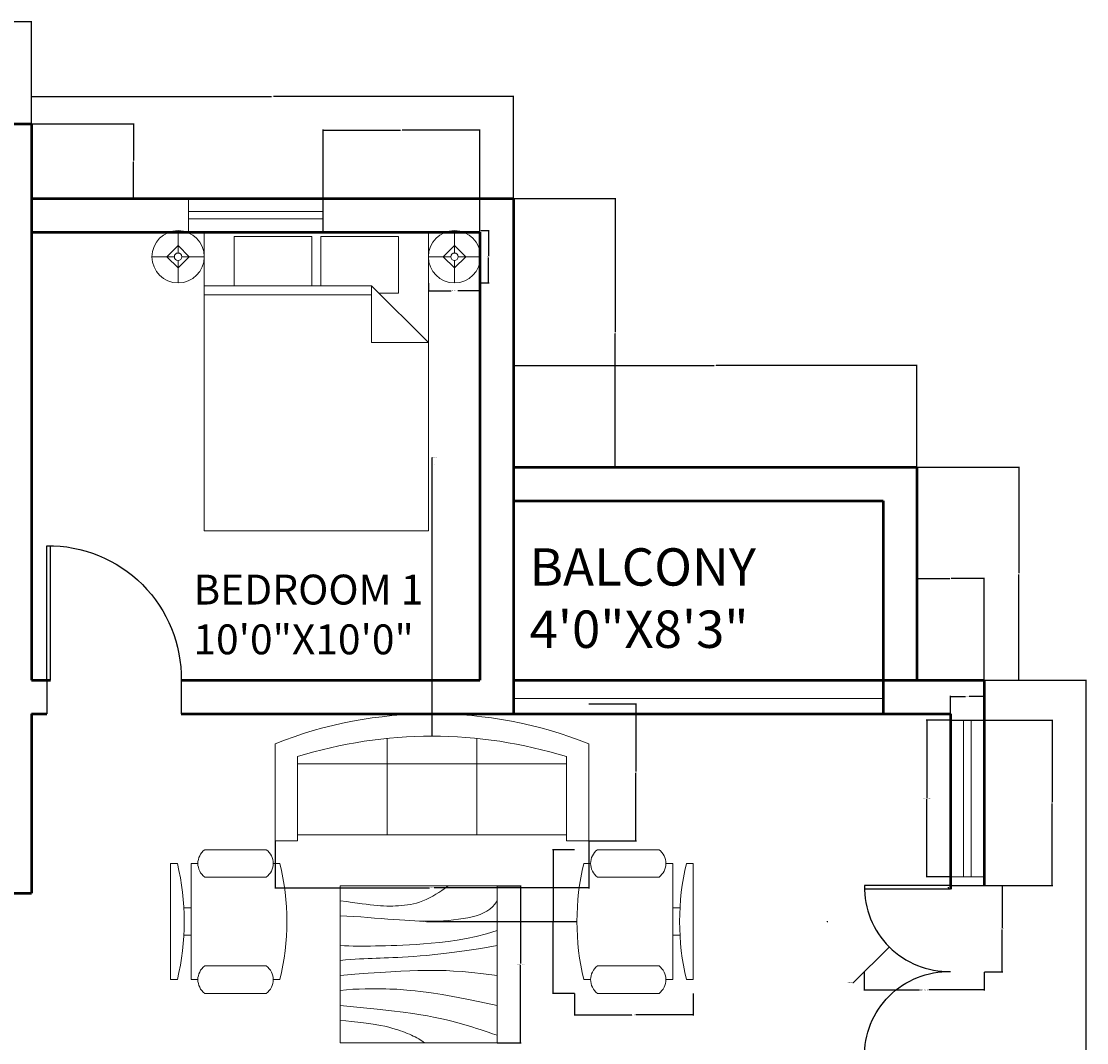
# Model space of a CAD drawing. Units: inches. Extents: x 178 to 719, y 262 to 748.
# Tile 3 of 3: x 434 to 719, y 475 to 748. Entities that reach past the tile are written whole.
import ezdxf

# ---------------------------------------------------------------- set-up
doc = ezdxf.new("R2010")
doc.units = ezdxf.units.IN
for name, color, linetype, lineweight in [('A-ANNO-DIMS', 2, 'Continuous', 18), ('A-AREA-IDEN', 7, 'Continuous', 25), ('A-DOOR', 3, 'Continuous', 25), ('A-FURN', 8, 'Continuous', 18), ('A-GLAZ', 4, 'Continuous', 18), ('A-WALL', 7, 'Continuous', 50)]:
    doc.layers.add(name, color=color, linetype=linetype, lineweight=lineweight)
doc.styles.get("Standard").update_dxf_attribs({"font": 'arial.ttf'})
doc.dimstyles.get("Standard").update_dxf_attribs({"dimtxt": 0.18, "dimasz": 0.18, "dimexe": 0.18, "dimexo": 0.0625, "dimgap": 0.09, "dimtad": 0, "dimtih": 1, "dimtoh": 1, "dimdec": 4, "dimzin": 0, "dimdsep": 46, "dimtxsty": 'Standard', "dimcen": 0.09, "dimadec": 0, "dimazin": 0, "dimtfac": 1, "dimtdec": 4, "dimtofl": 0, "dimtmove": 0, "dimatfit": 3, "dimfxl": 1, "dimtolj": 1, "dimtzin": 0, "dimarcsym": 0})

# ---------------------------------------------------------------- blocks, each defined once
blk = doc.blocks.new('Chair - Desk')
for p, q in [((-8.5, 0), (-8.5, -1)), ((-8.5, 0), (8.5, 0)), ((8.5, 0), (8.5, -1)), ((-8.5, -3), (-8.5, -4)), ((-8.5, -3), (8.5, -3)), ((-2, -3), (-2, -1.9355)), ((2, -1.9576), (2, -3)), ((8.5, -3), (8.5, -4)), ((-10.5, -5), (-10.5, -14)), ((-6.5, -14), (-6.5, -5)), ((6.5, -5), (6.5, -14)), ((10.5, -14), (10.5, -5)), ((-8.5, -15), (-8.5, -16)), ((8.5, -15), (8.5, -16))]:
    blk.add_line(p, q)
for centre, radius, start, end in [((0, 34.625), 36.625, 256.5803, 283.4197), ((-8.5, -6.5), 2.5, 36.8699, 143.1301), ((8.5, -6.5), 2.5, 36.8699, 143.1301), ((-8.5, -12.5), 2.5, 216.8699, 323.1301), ((8.5, -12.5), 2.5, 216.8699, 323.1301), ((0, 19.625), 36.625, 256.5803, 283.4197)]:
    blk.add_arc(centre, radius, start, end)
blk = doc.blocks.new('Sofa - Roundback 7 ft.')
for p, q in [((-12.00002, -32.4421), (-12.00003, -6.5971)), ((11.99997, -32.4421), (11.99998, -6.5971)), ((-36.000027, -34), (-36.000027, -11.4696)), ((-35.999844, -13.3819), (35.9998, -13.3819)), ((35.99998, -34), (35.99998, -11.4696)), ((-36.000027, -32.4421), (35.99998, -32.4421))]:
    blk.add_line(p, q)
for points in [[(-36.000027, -34), (-42.000027, -34), (-42.000027, -8)], [(41.99998, -8), (41.99998, -34), (35.99998, -34)]]:
    blk.add_lwpolyline(points)
for centre, radius, start, end in [((0, -114.25), 114.25, 68.43141, 111.5686), ((-0.00001, -127.1968), 121.1968, 72.72033, 107.2797)]:
    blk.add_arc(centre, radius, start, end)
blk = doc.blocks.new('Table - Square Woodgrain 42 x 42 in.')
blk.add_line((0, -42), (42, -42))
for points in [[(0, -4), (1.704, -4.2172), (3.2358, -4.4188), (4.615, -4.604), (5.8615, -4.7721), (6.9951, -4.9224), (8.0357, -5.0541), (9.0031, -5.1667), (9.9171, -5.2594), (10.7951, -5.3316), (11.6445, -5.3836), (12.4702, -5.4157), (13.277, -5.4283), (14.0698, -5.4217), (14.8535, -5.3964), (15.6331, -5.3526), (16.4133, -5.2908), (17.1986, -5.2103), (17.9913, -5.1062), (18.793, -4.9727), (19.6056, -4.8038), (20.4307, -4.5937), (21.2701, -4.3365), (22.1256, -4.0262), (22.9989, -3.6571), (23.888, -3.2272), (24.7756, -2.7516), (25.6408, -2.2491), (26.4624, -1.7387), (27.2195, -1.2395), (27.891, -0.7703), (28.456, -0.3501), (28.8934, 0.002)], [(0, -42), (0, 0), (42, 0), (42, -42)], [(0, -8), (1.8203, -8.1001), (3.6741, -8.2149), (5.5411, -8.3408), (7.4011, -8.4741), (9.2339, -8.6112), (11.0193, -8.7484), (12.7371, -8.8821), (14.3671, -9.0086), (15.8954, -9.1246), (17.3337, -9.2278), (18.6997, -9.3159), (20.0116, -9.387), (21.2871, -9.4389), (22.5442, -9.4696), (23.8008, -9.477), (25.0749, -9.459), (26.3791, -9.4137), (27.7049, -9.3403), (29.0383, -9.2382), (30.3655, -9.1068), (31.6728, -8.9455), (32.9461, -8.7535), (34.1717, -8.5304), (35.3358, -8.2756), (36.4268, -7.9863), (37.443, -7.6521), (38.3849, -7.2603), (39.253, -6.7986), (40.048, -6.2542), (40.7705, -5.6147), (41.421, -4.8674), (42, -4)], [(42, -12), (39.1784, -12.8621), (36.4519, -13.5654), (33.8246, -14.1294), (31.3004, -14.5731), (28.8832, -14.9161), (26.577, -15.1775), (24.3858, -15.3768), (22.3136, -15.5332), (20.3622, -15.6632), (18.5254, -15.7718), (16.7947, -15.8612), (15.1618, -15.9338), (13.6183, -15.9916), (12.1558, -16.0369), (10.7659, -16.0718), (9.4403, -16.0987), (8.1703, -16.1191), (6.9461, -16.1325), (5.7577, -16.1377), (4.595, -16.1335), (3.4479, -16.1188), (2.3064, -16.0924), (1.1604, -16.0532), (0, -16)], [(42, -16), (37.6529, -16.7365), (33.8802, -17.329), (30.6179, -17.7961), (27.8015, -18.1561), (25.3668, -18.4275), (23.2497, -18.6288), (21.3859, -18.7785), (19.7111, -18.8949), (18.1693, -18.9939), (16.7375, -19.0795), (15.401, -19.1534), (14.1449, -19.217), (12.9544, -19.2717), (11.8148, -19.3191), (10.7113, -19.3606), (9.6291, -19.3976), (8.5534, -19.4323), (7.47, -19.4689), (6.3643, -19.5122), (5.222, -19.5672), (4.0288, -19.6386), (2.7703, -19.7313), (1.4321, -19.8501), (0, -20)], [(0, -24), (3.9243, -23.6805), (7.4766, -23.4138), (10.6891, -23.1954), (13.5943, -23.0205), (16.2247, -22.8847), (18.6125, -22.7832), (20.7903, -22.7116), (22.7903, -22.6651), (24.6563, -22.642), (26.4764, -22.6507), (28.35, -22.7024), (30.3766, -22.8084), (32.6555, -22.98), (35.2861, -23.2283), (38.3678, -23.5645), (42, -24)], [(42, -32), (37.392, -31.017), (33.4585, -30.2231), (30.1291, -29.5949), (27.3334, -29.109), (25.0009, -28.742), (23.0612, -28.4707), (21.4439, -28.2716), (20.0786, -28.1215), (18.8998, -28.0002), (17.8609, -27.9014), (16.9206, -27.8219), (16.0371, -27.7588), (15.1691, -27.709), (14.2748, -27.6693), (13.3128, -27.6368), (12.2415, -27.6083), (11.0295, -27.5824), (9.6867, -27.5643), (8.233, -27.5608), (6.6884, -27.5787), (5.0728, -27.6248), (3.4062, -27.7058), (1.7086, -27.8286), (0, -28)], [(0, -32), (5.4026, -32.5358), (9.9494, -33.019), (13.7424, -33.4553), (16.8834, -33.8505), (19.4743, -34.2106), (21.6171, -34.5413), (23.4136, -34.8486), (24.9657, -35.1382), (26.3614, -35.4156), (27.6332, -35.6841), (28.7995, -35.9467), (29.8788, -36.2064), (30.8897, -36.4661), (31.8507, -36.7288), (32.7802, -36.9973), (33.6968, -37.2747), (34.6175, -37.5635), (35.5531, -37.8651), (36.5128, -38.1805), (37.506, -38.5108), (38.5421, -38.8568), (39.6302, -39.2197), (40.7797, -39.6004), (42, -40)], [(0, -36), (3.0098, -36.2857), (5.5354, -36.5643), (7.6368, -36.8359), (9.374, -37.1009), (10.807, -37.3597), (11.9957, -37.6126), (13.0002, -37.8599), (13.8804, -38.102), (14.6874, -38.3393), (15.4365, -38.5729), (16.1338, -38.8041), (16.7858, -39.0341), (17.3987, -39.264), (17.9787, -39.4952), (18.5322, -39.7288), (19.0655, -39.9662), (19.5832, -40.2081), (20.0842, -40.4544), (20.5657, -40.7046), (21.0249, -40.9581), (21.459, -41.2144), (21.8653, -41.4731), (22.2409, -41.7335), (22.5831, -41.9951)]]:
    blk.add_lwpolyline(points)
blk = doc.blocks.new('Bed - Queen')
for p, q in [((0, -80.00003), (0, 0)), ((0, 0), (59.99999, 0)), ((59.99999, 0), (59.99999, -80.00003)), ((7.99999, -1.2), (28.79998, -1.2)), ((7.99999, -14.4), (7.99999, -1.2)), ((28.79998, -1.2), (28.79998, -14.4)), ((31.19999, -1.2), (51.99999, -1.2)), ((31.19999, -14.4), (31.19999, -1.2)), ((51.99999, -1.2), (51.99999, -16.4)), ((0, -14.4), (44.8, -14.4)), ((44.8, -16.8), (0, -16.8)), ((59.99999, -29.6), (44.8, -14.4)), ((44.8, -14.4), (44.8, -29.6)), ((51.99999, -16.4), (46.79936, -16.4)), ((44.8, -29.6), (59.99999, -29.6)), ((59.99999, -80.00003), (0, -80.00003))]:
    blk.add_line(p, q)
blk = doc.blocks.new('Lamp - Table')
for p, q in [((0, 7), (0, 1)), ((0, 3), (-3, 0)), ((3, 0), (0, 3)), ((-1, 0), (-7, 0)), ((-3, 0), (0, -3)), ((0, -3), (3, 0)), ((1, 0), (7, 0)), ((0, -1), (0, -7))]:
    blk.add_line(p, q)
for radius in [7, 1]:
    blk.add_circle((0, 0), radius)
blk = doc.blocks.new('DOOR-SWING-36IN')
for p, q in [((-1, 0), (-1, 36)), ((0, 0), (0, 36)), ((-36, 0), (-36, -9)), ((0, 0), (0, -9))]:
    blk.add_line(p, q)
blk.add_arc((-0.5, 0.5), 35.5, 89.1931, 180.8069)
blk = doc.blocks.new('WINDOW-36IN')
for p, q in [((0, 0), (0, 9)), ((36, 0), (36, 9)), ((36, 5.5), (0, 5.5)), ((36, 3.5), (0, 3.5))]:
    blk.add_line(p, q)
blk = doc.blocks.new('WINDOW-42IN')
for p, q in [((0, 0), (-9, 0)), ((-5.5, 0), (-5.5, -42)), ((-3.5, 0), (-3.5, -36)), ((-3.5, 0), (-3.5, -36)), ((-3.5, 0), (-3.5, -42)), ((0, -42), (-9, -42))]:
    blk.add_line(p, q)
blk = doc.blocks.new('DOOR-PAIRED-LEAF-23IN')
for p, q in [((0, 0), (-23, 0)), ((0, 0), (9, 0)), ((0, -1), (-23, -1))]:
    blk.add_line(p, q)
blk.add_arc((-0.5, -0.5), 22.51, 178.727, 271.273)
blk = doc.blocks.new('*D17')
at = {"layer": 'A-ANNO-DIMS', "color": 0, "lineweight": -2, "transparency": 16777216}
for p, q in [((542.9, 678.05), (542.9, 675.84)), ((543.08, 676.02), (549, 676.02)), ((556.72, 676.02), (550.81, 676.02)), ((556.9, 678.05), (556.9, 675.84))]:
    blk.add_line(p, q, dxfattribs=at)
at = {"layer": 'A-ANNO-DIMS', "color": 0, "transparency": 16777216}
for points in [[(543.08, 676.05), (543.08, 675.99), (542.9, 676.02)], [(556.72, 676.05), (556.72, 675.99), (556.9, 676.02)]]:
    blk.add_solid(points, dxfattribs=at)
at = {"layer": 'Defpoints', "color": 0, "transparency": 16777216}
for p in [(542.9, 678.12), (556.9, 678.12), (556.9, 676.02)]:
    blk.add_point(p, dxfattribs=at)
at = {"layer": 'A-ANNO-DIMS', "color": 0, "transparency": 16777216, "insert": (549.9, 676.02), "char_height": 0.18, "attachment_point": 5}
blk.add_mtext('\\A1;LAMP 14 TYP.', dxfattribs=at)
blk = doc.blocks.new('*D18')
at = {"layer": 'A-ANNO-DIMS', "color": 0, "lineweight": -2, "transparency": 16777216}
for p, q in [((556.97, 692.12), (559.18, 692.12)), ((559, 691.94), (559, 685.3)), ((559, 678.3), (559, 684.94)), ((556.97, 678.12), (559.18, 678.12))]:
    blk.add_line(p, q, dxfattribs=at)
at = {"layer": 'A-ANNO-DIMS', "color": 0, "transparency": 16777216}
for points in [[(558.97, 691.94), (559.03, 691.94), (559, 692.12)], [(558.97, 678.3), (559.03, 678.3), (559, 678.12)]]:
    blk.add_solid(points, dxfattribs=at)
at = {"layer": 'Defpoints', "color": 0, "transparency": 16777216}
for p in [(556.9, 692.12), (559, 692.12), (556.9, 678.12)]:
    blk.add_point(p, dxfattribs=at)
at = {"layer": 'A-ANNO-DIMS', "color": 0, "transparency": 16777216, "insert": (559, 685.12), "char_height": 0.18, "attachment_point": 5}
blk.add_mtext('\\A1;14 TYP.', dxfattribs=at)
blk = doc.blocks.new('*D23')
at = {"layer": 'A-ANNO-DIMS', "color": 0, "lineweight": -2, "transparency": 16777216}
for p, q in [((659.56, 493.54), (659.56, 488.6)), ((691.7, 493.54), (691.7, 488.6)), ((659.74, 488.78), (674.35, 488.78)), ((691.52, 488.78), (676.92, 488.78))]:
    blk.add_line(p, q, dxfattribs=at)
at = {"layer": 'A-ANNO-DIMS', "color": 0, "transparency": 16777216}
for points in [[(659.74, 488.81), (659.74, 488.75), (659.56, 488.78)], [(691.52, 488.81), (691.52, 488.75), (691.7, 488.78)]]:
    blk.add_solid(points, dxfattribs=at)
at = {"layer": 'Defpoints', "color": 0, "transparency": 16777216}
for p in [(659.56, 493.6), (691.7, 493.6), (691.7, 488.78)]:
    blk.add_point(p, dxfattribs=at)
at = {"layer": 'A-ANNO-DIMS', "color": 0, "transparency": 16777216, "insert": (675.63, 488.78), "char_height": 0.18, "attachment_point": 5}
blk.add_mtext('\\A1;DOOR LEAF 32 TYP.', dxfattribs=at)
blk = doc.blocks.new('*D24')
at = {"layer": 'A-ANNO-DIMS', "color": 0, "lineweight": -2, "transparency": 16777216}
for p, q in [((691.76, 516.74), (696.7, 516.74)), ((696.52, 516.56), (696.52, 505.35)), ((696.52, 493.78), (696.52, 504.99)), ((691.76, 493.6), (696.7, 493.6))]:
    blk.add_line(p, q, dxfattribs=at)
at = {"layer": 'A-ANNO-DIMS', "color": 0, "transparency": 16777216}
for points in [[(696.49, 516.56), (696.55, 516.56), (696.52, 516.74)], [(696.49, 493.78), (696.55, 493.78), (696.52, 493.6)]]:
    blk.add_solid(points, dxfattribs=at)
at = {"layer": 'Defpoints', "color": 0, "transparency": 16777216}
for p in [(691.7, 516.74), (696.52, 516.74), (691.7, 493.6)]:
    blk.add_point(p, dxfattribs=at)
at = {"layer": 'A-ANNO-DIMS', "color": 0, "transparency": 16777216, "insert": (696.52, 505.17), "char_height": 0.18, "attachment_point": 5}
blk.add_mtext('\\A1;23 TYP.', dxfattribs=at)
blk = doc.blocks.new('*D27')
at = {"layer": 'A-ANNO-DIMS', "color": 0, "lineweight": -2, "transparency": 16777216}
for p, q in [((682.64, 561.07), (676.22, 561.07)), ((676.4, 560.89), (676.4, 540.26)), ((676.4, 519.25), (676.4, 539.89)), ((682.64, 519.07), (676.22, 519.07))]:
    blk.add_line(p, q, dxfattribs=at)
at = {"layer": 'A-ANNO-DIMS', "color": 0, "transparency": 16777216}
for points in [[(676.37, 560.89), (676.43, 560.89), (676.4, 561.07)], [(676.37, 519.25), (676.43, 519.25), (676.4, 519.07)]]:
    blk.add_solid(points, dxfattribs=at)
at = {"layer": 'Defpoints', "color": 0, "transparency": 16777216}
for p in [(676.4, 561.07), (682.7, 561.07), (682.7, 519.07)]:
    blk.add_point(p, dxfattribs=at)
at = {"layer": 'A-ANNO-DIMS', "color": 0, "transparency": 16777216, "insert": (676.4, 540.07), "char_height": 0.18, "attachment_point": 5}
blk.add_mtext('\\A1;WINDOW 42 TYP.', dxfattribs=at)
blk = doc.blocks.new('*D28')
at = {"layer": 'A-ANNO-DIMS', "color": 0, "lineweight": -2, "transparency": 16777216}
for p, q in [((682.7, 561.14), (682.7, 567.55)), ((682.88, 567.37), (686.74, 567.37)), ((691.52, 567.37), (687.66, 567.37)), ((691.7, 561.14), (691.7, 567.55))]:
    blk.add_line(p, q, dxfattribs=at)
at = {"layer": 'A-ANNO-DIMS', "color": 0, "transparency": 16777216}
for points in [[(682.88, 567.4), (682.88, 567.34), (682.7, 567.37)], [(691.52, 567.4), (691.52, 567.34), (691.7, 567.37)]]:
    blk.add_solid(points, dxfattribs=at)
at = {"layer": 'Defpoints', "color": 0, "transparency": 16777216}
for p in [(691.7, 567.37), (682.7, 561.07), (691.7, 561.07)]:
    blk.add_point(p, dxfattribs=at)
at = {"layer": 'A-ANNO-DIMS', "color": 0, "transparency": 16777216, "insert": (687.2, 567.37), "char_height": 0.18, "attachment_point": 5}
blk.add_mtext('\\A1;9 TYP.', dxfattribs=at)
blk = doc.blocks.new('*D33')
at = {"layer": 'A-ANNO-DIMS', "color": 0, "lineweight": -2, "transparency": 16777216}
for p, q in [((582.01, 526.35), (576.12, 526.35)), ((576.3, 526.17), (576.3, 507.3)), ((576.3, 488.06), (576.3, 506.93)), ((582.01, 487.88), (576.12, 487.88))]:
    blk.add_line(p, q, dxfattribs=at)
at = {"layer": 'A-ANNO-DIMS', "color": 0, "transparency": 16777216}
for points in [[(576.27, 526.17), (576.33, 526.17), (576.3, 526.35)], [(576.27, 488.06), (576.33, 488.06), (576.3, 487.88)]]:
    blk.add_solid(points, dxfattribs=at)
at = {"layer": 'Defpoints', "color": 0, "transparency": 16777216}
for p in [(582.07, 526.35), (576.3, 487.88), (582.07, 487.88)]:
    blk.add_point(p, dxfattribs=at)
at = {"layer": 'A-ANNO-DIMS', "color": 0, "transparency": 16777216, "insert": (576.3, 507.12), "char_height": 0.18, "attachment_point": 5}
blk.add_mtext('\\A1;CHAIR 38 TYP.', dxfattribs=at)
blk = doc.blocks.new('*D34')
at = {"layer": 'A-ANNO-DIMS', "color": 0, "lineweight": -2, "transparency": 16777216}
for p, q in [((582.07, 487.82), (582.07, 481.93)), ((613.82, 487.82), (613.82, 481.93)), ((582.25, 482.11), (597.42, 482.11)), ((613.64, 482.11), (598.48, 482.11))]:
    blk.add_line(p, q, dxfattribs=at)
at = {"layer": 'A-ANNO-DIMS', "color": 0, "transparency": 16777216}
for points in [[(582.25, 482.14), (582.25, 482.08), (582.07, 482.11)], [(613.64, 482.14), (613.64, 482.08), (613.82, 482.11)]]:
    blk.add_solid(points, dxfattribs=at)
at = {"layer": 'Defpoints', "color": 0, "transparency": 16777216}
for p in [(582.07, 487.88), (613.82, 487.88), (613.82, 482.11)]:
    blk.add_point(p, dxfattribs=at)
at = {"layer": 'A-ANNO-DIMS', "color": 0, "transparency": 16777216, "insert": (597.95, 482.11), "char_height": 0.18, "attachment_point": 5}
blk.add_mtext('\\A1;32 TYP.', dxfattribs=at)
blk = doc.blocks.new('*D37')
at = {"layer": 'A-ANNO-DIMS', "color": 0, "lineweight": -2, "transparency": 16777216}
for p, q in [((501.85, 528.67), (501.85, 515.96)), ((585.85, 528.67), (585.85, 515.96)), ((502.03, 516.14), (543.25, 516.14)), ((585.67, 516.14), (544.44, 516.14))]:
    blk.add_line(p, q, dxfattribs=at)
at = {"layer": 'A-ANNO-DIMS', "color": 0, "transparency": 16777216}
for points in [[(502.03, 516.17), (502.03, 516.11), (501.85, 516.14)], [(585.67, 516.17), (585.67, 516.11), (585.85, 516.14)]]:
    blk.add_solid(points, dxfattribs=at)
at = {"layer": 'Defpoints', "color": 0, "transparency": 16777216}
for p in [(501.85, 528.74), (585.85, 528.74), (585.85, 516.14)]:
    blk.add_point(p, dxfattribs=at)
at = {"layer": 'A-ANNO-DIMS', "color": 0, "transparency": 16777216, "insert": (543.85, 516.14), "char_height": 0.18, "attachment_point": 5}
blk.add_mtext('\\A1;SOFA 84', dxfattribs=at)
blk = doc.blocks.new('*D38')
at = {"layer": 'A-ANNO-DIMS', "color": 0, "lineweight": -2, "transparency": 16777216}
for p, q in [((585.91, 565.4), (598.63, 565.4)), ((598.45, 565.22), (598.45, 547.25)), ((598.45, 528.92), (598.45, 546.89)), ((585.91, 528.74), (598.63, 528.74))]:
    blk.add_line(p, q, dxfattribs=at)
at = {"layer": 'A-ANNO-DIMS', "color": 0, "transparency": 16777216}
for points in [[(598.42, 565.22), (598.48, 565.22), (598.45, 565.4)], [(598.42, 528.92), (598.48, 528.92), (598.45, 528.74)]]:
    blk.add_solid(points, dxfattribs=at)
at = {"layer": 'Defpoints', "color": 0, "transparency": 16777216}
for p in [(585.85, 565.4), (598.45, 565.4), (585.85, 528.74)]:
    blk.add_point(p, dxfattribs=at)
at = {"layer": 'A-ANNO-DIMS', "color": 0, "transparency": 16777216, "insert": (598.45, 547.07), "char_height": 0.18, "attachment_point": 5}
blk.add_mtext('\\A1;37', dxfattribs=at)
blk = doc.blocks.new('*D39')
at = {"layer": 'A-ANNO-DIMS', "color": 0, "lineweight": -2, "transparency": 16777216}
for p, q in [((561.35, 516.67), (567.77, 516.67)), ((567.59, 516.49), (567.59, 495.85)), ((567.59, 474.85), (567.59, 495.49)), ((561.35, 474.67), (567.77, 474.67))]:
    blk.add_line(p, q, dxfattribs=at)
at = {"layer": 'A-ANNO-DIMS', "color": 0, "transparency": 16777216}
for points in [[(567.56, 516.49), (567.62, 516.49), (567.59, 516.67)], [(567.56, 474.85), (567.62, 474.85), (567.59, 474.67)]]:
    blk.add_solid(points, dxfattribs=at)
at = {"layer": 'Defpoints', "color": 0, "transparency": 16777216}
for p in [(561.29, 516.67), (567.59, 516.67), (561.29, 474.67)]:
    blk.add_point(p, dxfattribs=at)
at = {"layer": 'A-ANNO-DIMS', "color": 0, "transparency": 16777216, "insert": (567.59, 495.67), "char_height": 0.18, "attachment_point": 5}
blk.add_mtext('\\A1;COFFEE TABLE 42', dxfattribs=at)
blk = doc.blocks.new('*D44')
at = {"layer": 'A-ANNO-DIMS', "color": 0, "lineweight": -2, "transparency": 16777216}
for p, q in [((223.7, 720.8), (223.7, 748.17)), ((223.88, 747.99), (329.91, 747.99)), ((436.52, 747.99), (330.49, 747.99)), ((436.7, 720.8), (436.7, 748.17))]:
    blk.add_line(p, q, dxfattribs=at)
at = {"layer": 'A-ANNO-DIMS', "color": 0, "transparency": 16777216}
for points in [[(223.88, 748.02), (223.88, 747.96), (223.7, 747.99)], [(436.52, 748.02), (436.52, 747.96), (436.7, 747.99)]]:
    blk.add_solid(points, dxfattribs=at)
at = {"layer": 'Defpoints', "color": 0, "transparency": 16777216}
for p in [(436.7, 747.99), (223.7, 720.74), (436.7, 720.74)]:
    blk.add_point(p, dxfattribs=at)
at = {"layer": 'A-ANNO-DIMS', "color": 0, "transparency": 16777216, "insert": (330.2, 747.99), "char_height": 0.18, "attachment_point": 5}
blk.add_mtext('\\A1;213', dxfattribs=at)
blk = doc.blocks.new('*D45')
at = {"layer": 'A-ANNO-DIMS', "color": 0, "lineweight": -2, "transparency": 16777216}
for p, q in [((565.7, 628.8), (565.7, 656.17)), ((673.7, 628.8), (673.7, 656.17)), ((565.88, 655.99), (619.42, 655.99)), ((673.52, 655.99), (619.98, 655.99))]:
    blk.add_line(p, q, dxfattribs=at)
at = {"layer": 'A-ANNO-DIMS', "color": 0, "transparency": 16777216}
for points in [[(565.88, 656.02), (565.88, 655.96), (565.7, 655.99)], [(673.52, 656.02), (673.52, 655.96), (673.7, 655.99)]]:
    blk.add_solid(points, dxfattribs=at)
at = {"layer": 'Defpoints', "color": 0, "transparency": 16777216}
for p in [(673.7, 655.99), (565.7, 628.74), (673.7, 628.74)]:
    blk.add_point(p, dxfattribs=at)
at = {"layer": 'A-ANNO-DIMS', "color": 0, "transparency": 16777216, "insert": (619.7, 655.99), "char_height": 0.18, "attachment_point": 5}
blk.add_mtext('\\A1;108', dxfattribs=at)
blk = doc.blocks.new('*D46')
at = {"layer": 'A-ANNO-DIMS', "color": 0, "lineweight": -2, "transparency": 16777216}
for p, q in [((436.7, 700.8), (436.7, 728.17)), ((436.88, 727.99), (500.92, 727.99)), ((565.52, 727.99), (501.48, 727.99)), ((565.7, 700.8), (565.7, 728.17))]:
    blk.add_line(p, q, dxfattribs=at)
at = {"layer": 'A-ANNO-DIMS', "color": 0, "transparency": 16777216}
for points in [[(436.88, 728.02), (436.88, 727.96), (436.7, 727.99)], [(565.52, 728.02), (565.52, 727.96), (565.7, 727.99)]]:
    blk.add_solid(points, dxfattribs=at)
at = {"layer": 'Defpoints', "color": 0, "transparency": 16777216}
for p in [(565.7, 727.99), (436.7, 700.74), (565.7, 700.74)]:
    blk.add_point(p, dxfattribs=at)
at = {"layer": 'A-ANNO-DIMS', "color": 0, "transparency": 16777216, "insert": (501.2, 727.99), "char_height": 0.18, "attachment_point": 5}
blk.add_mtext('\\A1;129', dxfattribs=at)
blk = doc.blocks.new('*D47')
at = {"layer": 'A-ANNO-DIMS', "color": 0, "lineweight": -2, "transparency": 16777216}
for p, q in [((673.7, 571.8), (673.7, 599.17)), ((673.88, 598.99), (682.49, 598.99)), ((691.52, 598.99), (682.91, 598.99)), ((691.7, 571.8), (691.7, 599.17))]:
    blk.add_line(p, q, dxfattribs=at)
at = {"layer": 'A-ANNO-DIMS', "color": 0, "transparency": 16777216}
for points in [[(673.88, 599.02), (673.88, 598.96), (673.7, 598.99)], [(691.52, 599.02), (691.52, 598.96), (691.7, 598.99)]]:
    blk.add_solid(points, dxfattribs=at)
at = {"layer": 'Defpoints', "color": 0, "transparency": 16777216}
for p in [(691.7, 598.99), (673.7, 571.74), (691.7, 571.74)]:
    blk.add_point(p, dxfattribs=at)
at = {"layer": 'A-ANNO-DIMS', "color": 0, "transparency": 16777216, "insert": (682.7, 598.99), "char_height": 0.18, "attachment_point": 5}
blk.add_mtext('\\A1;18', dxfattribs=at)
blk = doc.blocks.new('*D49')
at = {"layer": 'A-ANNO-DIMS', "color": 0, "lineweight": -2, "transparency": 16777216}
for p, q in [((691.76, 571.74), (719.13, 571.74)), ((718.95, 571.56), (718.95, 466.92)), ((718.95, 361.92), (718.95, 466.56)), ((691.76, 361.74), (719.13, 361.74))]:
    blk.add_line(p, q, dxfattribs=at)
at = {"layer": 'A-ANNO-DIMS', "color": 0, "transparency": 16777216}
for points in [[(718.92, 571.56), (718.98, 571.56), (718.95, 571.74)], [(718.92, 361.92), (718.98, 361.92), (718.95, 361.74)]]:
    blk.add_solid(points, dxfattribs=at)
at = {"layer": 'Defpoints', "color": 0, "transparency": 16777216}
for p in [(691.7, 571.74), (691.7, 361.74), (718.95, 361.74)]:
    blk.add_point(p, dxfattribs=at)
at = {"layer": 'A-ANNO-DIMS', "color": 0, "transparency": 16777216, "insert": (718.95, 466.74), "char_height": 0.18, "attachment_point": 5}
blk.add_mtext('\\A1;210', dxfattribs=at)
blk = doc.blocks.new('*D50')
at = {"layer": 'A-ANNO-DIMS', "color": 0, "lineweight": -2, "transparency": 16777216}
for p, q in [((673.76, 628.74), (701.13, 628.74)), ((700.95, 628.56), (700.95, 600.42)), ((700.95, 571.92), (700.95, 600.06)), ((673.76, 571.74), (701.13, 571.74))]:
    blk.add_line(p, q, dxfattribs=at)
at = {"layer": 'A-ANNO-DIMS', "color": 0, "transparency": 16777216}
for points in [[(700.92, 628.56), (700.98, 628.56), (700.95, 628.74)], [(700.92, 571.92), (700.98, 571.92), (700.95, 571.74)]]:
    blk.add_solid(points, dxfattribs=at)
at = {"layer": 'Defpoints', "color": 0, "transparency": 16777216}
for p in [(673.7, 628.74), (673.7, 571.74), (700.95, 571.74)]:
    blk.add_point(p, dxfattribs=at)
at = {"layer": 'A-ANNO-DIMS', "color": 0, "transparency": 16777216, "insert": (700.95, 600.24), "char_height": 0.18, "attachment_point": 5}
blk.add_mtext('\\A1;57', dxfattribs=at)
blk = doc.blocks.new('*D51')
at = {"layer": 'A-ANNO-DIMS', "color": 0, "lineweight": -2, "transparency": 16777216}
for p, q in [((565.76, 700.74), (593.13, 700.74)), ((592.95, 700.56), (592.95, 664.92)), ((592.95, 628.92), (592.95, 664.56)), ((565.76, 628.74), (593.13, 628.74))]:
    blk.add_line(p, q, dxfattribs=at)
at = {"layer": 'A-ANNO-DIMS', "color": 0, "transparency": 16777216}
for points in [[(592.92, 700.56), (592.98, 700.56), (592.95, 700.74)], [(592.92, 628.92), (592.98, 628.92), (592.95, 628.74)]]:
    blk.add_solid(points, dxfattribs=at)
at = {"layer": 'Defpoints', "color": 0, "transparency": 16777216}
for p in [(565.7, 700.74), (565.7, 628.74), (592.95, 628.74)]:
    blk.add_point(p, dxfattribs=at)
at = {"layer": 'A-ANNO-DIMS', "color": 0, "transparency": 16777216, "insert": (592.95, 664.74), "char_height": 0.18, "attachment_point": 5}
blk.add_mtext('\\A1;72', dxfattribs=at)
blk = doc.blocks.new('*D52')
at = {"layer": 'A-ANNO-DIMS', "color": 0, "lineweight": -2, "transparency": 16777216}
for p, q in [((436.76, 720.74), (464.13, 720.74)), ((463.95, 720.56), (463.95, 710.92)), ((463.95, 700.92), (463.95, 710.56)), ((436.76, 700.74), (464.13, 700.74))]:
    blk.add_line(p, q, dxfattribs=at)
at = {"layer": 'A-ANNO-DIMS', "color": 0, "transparency": 16777216}
for points in [[(463.92, 720.56), (463.98, 720.56), (463.95, 720.74)], [(463.92, 700.92), (463.98, 700.92), (463.95, 700.74)]]:
    blk.add_solid(points, dxfattribs=at)
at = {"layer": 'Defpoints', "color": 0, "transparency": 16777216}
for p in [(436.7, 720.74), (436.7, 700.74), (463.95, 700.74)]:
    blk.add_point(p, dxfattribs=at)
at = {"layer": 'A-ANNO-DIMS', "color": 0, "transparency": 16777216, "insert": (463.95, 710.74), "char_height": 0.18, "attachment_point": 5}
blk.add_mtext('\\A1;20', dxfattribs=at)
blk = doc.blocks.new('*D58')
at = {"layer": 'A-ANNO-DIMS', "color": 0, "lineweight": -2, "transparency": 16777216}
for p, q in [((514.7, 691.8), (514.7, 719.17)), ((514.88, 718.99), (535.48, 718.99)), ((556.52, 718.99), (535.92, 718.99)), ((556.7, 691.8), (556.7, 719.17))]:
    blk.add_line(p, q, dxfattribs=at)
at = {"layer": 'A-ANNO-DIMS', "color": 0, "transparency": 16777216}
for points in [[(514.88, 719.02), (514.88, 718.96), (514.7, 718.99)], [(556.52, 719.02), (556.52, 718.96), (556.7, 718.99)]]:
    blk.add_solid(points, dxfattribs=at)
at = {"layer": 'Defpoints', "color": 0, "transparency": 16777216}
for p in [(556.7, 718.99), (514.7, 691.74), (556.7, 691.74)]:
    blk.add_point(p, dxfattribs=at)
at = {"layer": 'A-ANNO-DIMS', "color": 0, "transparency": 16777216, "insert": (535.7, 718.99), "char_height": 0.18, "attachment_point": 5}
blk.add_mtext('\\A1;42', dxfattribs=at)
blk = doc.blocks.new('*D63')
at = {"layer": 'A-ANNO-DIMS', "color": 0, "lineweight": -2, "transparency": 16777216}
for p, q in [((682.76, 561.07), (710.13, 561.07)), ((709.95, 560.89), (709.95, 539.09)), ((709.95, 516.92), (709.95, 538.72)), ((682.76, 516.74), (710.13, 516.74))]:
    blk.add_line(p, q, dxfattribs=at)
at = {"layer": 'A-ANNO-DIMS', "color": 0, "transparency": 16777216}
for points in [[(709.92, 560.89), (709.98, 560.89), (709.95, 561.07)], [(709.92, 516.92), (709.98, 516.92), (709.95, 516.74)]]:
    blk.add_solid(points, dxfattribs=at)
at = {"layer": 'Defpoints', "color": 0, "transparency": 16777216}
for p in [(682.7, 561.07), (682.7, 516.74), (709.95, 516.74)]:
    blk.add_point(p, dxfattribs=at)
at = {"layer": 'A-ANNO-DIMS', "color": 0, "transparency": 16777216, "insert": (709.95, 538.91), "char_height": 0.18, "attachment_point": 5}
blk.add_mtext('\\A1;44.34', dxfattribs=at)
blk = doc.blocks.new('*D72')
at = {"layer": 'A-ANNO-DIMS', "color": 0, "lineweight": -2, "transparency": 16777216}
for p, q in [((682.2, 516.15), (682.2, 516.33)), ((682.11, 516.24), (682.29, 516.24)), ((656.74, 490.77), (666.16, 500.2)), ((656.56, 490.77), (656.74, 490.77))]:
    blk.add_line(p, q, dxfattribs=at)
at = {"layer": 'A-ANNO-DIMS', "color": 0, "transparency": 16777216}
blk.add_solid([(666.14, 500.22), (666.18, 500.17), (666.29, 500.32)], dxfattribs=at)
at = {"layer": 'Defpoints', "color": 0, "transparency": 16777216}
for p in [(682.2, 516.24), (666.29, 500.32)]:
    blk.add_point(p, dxfattribs=at)
at = {"layer": 'A-ANNO-DIMS', "color": 0, "transparency": 16777216, "insert": (655.81, 490.77), "char_height": 0.18, "attachment_point": 5}
blk.add_mtext('\\A1;2X R22.506', dxfattribs=at)
blk = doc.blocks.new('*D73')
at = {"layer": 'A-ANNO-DIMS', "color": 0, "lineweight": -2, "transparency": 16777216}
for p, q in [((544.03, 629.46), (543.85, 629.46)), ((543.85, 629.46), (543.85, 556.92)), ((543.76, 435.54), (543.94, 435.54)), ((543.85, 435.45), (543.85, 435.63))]:
    blk.add_line(p, q, dxfattribs=at)
at = {"layer": 'A-ANNO-DIMS', "color": 0, "transparency": 16777216}
blk.add_solid([(543.82, 556.92), (543.88, 556.92), (543.85, 556.74)], dxfattribs=at)
at = {"layer": 'Defpoints', "color": 0, "transparency": 16777216}
for p in [(543.85, 556.74), (543.85, 435.54)]:
    blk.add_point(p, dxfattribs=at)
at = {"layer": 'A-ANNO-DIMS', "color": 0, "transparency": 16777216, "insert": (544.51, 629.46), "char_height": 0.18, "attachment_point": 5}
blk.add_mtext('\\A1;R121.2', dxfattribs=at)
blk = doc.blocks.new('*D74')
at = {"layer": 'A-ANNO-DIMS', "color": 0, "lineweight": -2, "transparency": 16777216}
for p, q in [((544.03, 631.29), (543.85, 631.29)), ((543.85, 631.29), (543.85, 562.92)), ((543.76, 448.49), (543.94, 448.49)), ((543.85, 448.4), (543.85, 448.58))]:
    blk.add_line(p, q, dxfattribs=at)
at = {"layer": 'A-ANNO-DIMS', "color": 0, "transparency": 16777216}
blk.add_solid([(543.82, 562.92), (543.88, 562.92), (543.85, 562.74)], dxfattribs=at)
at = {"layer": 'Defpoints', "color": 0, "transparency": 16777216}
for p in [(543.85, 562.74), (543.85, 448.49)]:
    blk.add_point(p, dxfattribs=at)
at = {"layer": 'A-ANNO-DIMS', "color": 0, "transparency": 16777216, "insert": (544.58, 631.29), "char_height": 0.18, "attachment_point": 5}
blk.add_mtext('\\A1;R114.25', dxfattribs=at)
blk = doc.blocks.new('*D75')
at = {"layer": 'A-ANNO-DIMS', "color": 0, "lineweight": -2, "transparency": 16777216}
for p, q in [((542.42, 507.12), (582.5, 507.12)), ((649.69, 507.12), (649.87, 507.12)), ((649.78, 507.03), (649.78, 507.21))]:
    blk.add_line(p, q, dxfattribs=at)
at = {"layer": 'A-ANNO-DIMS', "color": 0, "transparency": 16777216}
blk.add_solid([(582.5, 507.15), (582.5, 507.09), (582.68, 507.12)], dxfattribs=at)
at = {"layer": 'Defpoints', "color": 0, "transparency": 16777216}
for p in [(582.68, 507.12), (649.78, 507.12)]:
    blk.add_point(p, dxfattribs=at)
at = {"layer": 'A-ANNO-DIMS', "color": 0, "transparency": 16777216, "insert": (541.84, 507.12), "char_height": 0.18, "attachment_point": 5}
blk.add_mtext('\\A1;4X R67.1', dxfattribs=at)

msp = doc.modelspace()

# ---------------------------------------------------------------- linework, layer by layer
at = {"layer": 'A-GLAZ'}
msp.add_line((565.7008, 566.8715), (664.7008, 566.8715), dxfattribs=at)
at = {"layer": 'A-WALL'}
for p, q in [((295.7008, 720.737), (436.7008, 720.737)), ((436.7008, 720.737), (436.7008, 571.737)), ((436.7008, 700.737), (565.7008, 700.737)), ((565.7008, 700.737), (565.7008, 562.737)), ((436.7008, 691.737), (556.7008, 691.737)), ((556.7008, 691.737), (556.7008, 571.737)), ((565.7008, 628.737), (673.7008, 628.737)), ((673.7008, 628.737), (673.7008, 571.737)), ((565.7008, 619.737), (664.7008, 619.737)), ((664.7008, 619.737), (664.7008, 562.737)), ((436.7008, 571.737), (441.7397, 571.737)), ((476.7397, 571.737), (556.7008, 571.737)), ((565.7008, 571.737), (691.7008, 571.737)), ((691.7008, 571.737), (691.7008, 516.737)), ((436.7008, 562.737), (440.7397, 562.737)), ((436.7008, 562.737), (436.7008, 514.737)), ((476.7397, 562.737), (682.7008, 562.737)), ((682.7008, 562.737), (682.7008, 515.737)), ((423.2008, 514.737), (436.7008, 514.737))]:
    msp.add_line(p, q, dxfattribs=at)

# ---------------------------------------------------------------- block references
at = {"layer": 'A-DOOR', "extrusion": (0, 0, -1), "zscale": -1}
msp.add_blockref('DOOR-SWING-36IN', (-440.7397, 571.737), dxfattribs=at)
at = {"layer": 'A-DOOR'}
msp.add_blockref('DOOR-PAIRED-LEAF-23IN', (682.7008, 516.737), dxfattribs=at)
at = {"layer": 'A-DOOR', "extrusion": (0, 0, -1), "zscale": -1, "rotation": 180}
msp.add_blockref('DOOR-PAIRED-LEAF-23IN', (-682.7008, 470.737), dxfattribs=at)
at = {"layer": 'A-FURN'}
for name, p in [('Lamp - Table', (475.9072, 685.1157)), ('Bed - Queen', (482.9044, 691.737)), ('Lamp - Table', (549.9044, 685.1157)), ('Sofa - Roundback 7 ft.', (543.8486, 562.737)), ('Table - Square Woodgrain 42 x 42 in.', (519.289, 516.6678))]:
    msp.add_blockref(name, p, dxfattribs=at)
at = {"layer": 'A-FURN', "yscale": 1.831941339206794, "zscale": 1.831941339206794}
for p, xscale, rotation in [((473.8723, 507.1176), -1.831941339206794, 90), ((613.8249, 507.1176), 1.831941339206794, 270)]:
    msp.add_blockref('Chair - Desk', p, dxfattribs=dict(at, xscale=xscale, rotation=rotation))
at = {"layer": 'A-GLAZ'}
for name, p in [('WINDOW-36IN', (478.7008, 691.737)), ('WINDOW-42IN', (691.7008, 561.0742))]:
    msp.add_blockref(name, p, dxfattribs=at)

# ---------------------------------------------------------------- texts
at = {"layer": 'A-AREA-IDEN', "attachment_point": 1}
for s, insert, char_height in [('BALCONY\\P4\'0"X8\'3"', (570, 607.0555), 10), ('BEDROOM 1\\P10\'0"X10\'0"', (480, 600), 8)]:
    msp.add_mtext_dynamic_manual_height_columns(s, width=98.987328, gutter_width=12.5, heights=[0], dxfattribs=dict(at, insert=insert, char_height=char_height))

# ---------------------------------------------------------------- dimensions: what is measured, and where the dimension line sits
at = {"layer": 'A-ANNO-DIMS'}
for base, p1, p2, picture, middle in [((436.7008, 747.987), (223.7008, 720.737), (436.7008, 720.737), '*D44', (330.2008, 747.987)), ((673.7008, 655.987), (565.7008, 628.737), (673.7008, 628.737), '*D45', (619.7008, 655.987)), ((691.7008, 598.987), (673.7008, 571.737), (691.7008, 571.737), '*D47', (682.7008, 598.987))]:
    dim = msp.add_linear_dim(base=base, p1=p1, p2=p2, dimstyle='Standard', override={"dimdec": 0, "dimlfac": 1, "dimrnd": 0, "dimzin": 0, "dimdsep": 46, "dimlunit": 2}, dxfattribs=at)
    dim.commit()
    dim.dimension.update_dxf_attribs({"geometry": picture, "text_midpoint": middle})
for base, p1, p2, angle, override, picture, middle in [((565.7008, 727.987), (436.7008, 700.737), (565.7008, 700.737), 0, {"dimdec": 0, "dimlfac": 1, "dimrnd": 0, "dimzin": 0, "dimdsep": 46, "dimlunit": 2}, '*D46', (501.2008, 727.987)), ((463.9508, 700.737), (436.7008, 720.737), (436.7008, 700.737), 270, {"dimdec": 0, "dimlfac": 1, "dimrnd": 0, "dimzin": 0, "dimdsep": 46, "dimlunit": 2}, '*D52', (463.9508, 710.737)), ((556.7008, 718.987), (514.7008, 691.737), (556.7008, 691.737), 0, {"dimdec": 0, "dimlfac": 1, "dimrnd": 0, "dimzin": 0, "dimdsep": 46, "dimlunit": 2}, '*D58', (535.7008, 718.987)), ((592.9508, 628.737), (565.7008, 700.737), (565.7008, 628.737), 270, {"dimdec": 0, "dimlfac": 1, "dimrnd": 0, "dimzin": 0, "dimdsep": 46, "dimlunit": 2}, '*D51', (592.9508, 664.737)), ((700.9508, 571.737), (673.7008, 628.737), (673.7008, 571.737), 270, {"dimdec": 0, "dimlfac": 1, "dimrnd": 0, "dimzin": 0, "dimdsep": 46, "dimlunit": 2}, '*D50', (700.9508, 600.237)), ((718.9508, 361.737), (691.7008, 571.737), (691.7008, 361.737), 270, {"dimdec": 0, "dimlfac": 1, "dimrnd": 0, "dimzin": 0, "dimdsep": 46, "dimlunit": 2}, '*D49', (718.9508, 466.737)), ((598.4486, 565.4037), (585.8486, 528.737), (585.8486, 565.4037), 90, {"dimdec": 0, "dimlfac": 1, "dimrnd": 0, "dimzin": 0, "dimdsep": 46, "dimlunit": 2}, '*D38', (598.4486, 547.0703)), ((709.9508, 516.737), (682.7008, 561.0742), (682.7008, 516.737), 270, {"dimdec": 2, "dimlfac": 1, "dimrnd": 0, "dimzin": 0, "dimdsep": 46, "dimlunit": 2}, '*D63', (709.9508, 538.9056))]:
    dim = msp.add_linear_dim(base=base, p1=p1, p2=p2, angle=angle, dimstyle='Standard', override=override, dxfattribs=at)
    dim.commit()
    dim.dimension.update_dxf_attribs({"geometry": picture, "text_midpoint": middle})
for base, p1, p2, angle, text, picture, middle in [((559.0044, 692.1157), (556.9044, 678.1157), (556.9044, 692.1157), 90, '<> TYP.', '*D18', (559.0044, 685.1157)), ((676.4008, 561.0742), (682.7008, 519.0742), (682.7008, 561.0742), 90, 'WINDOW <> TYP.', '*D27', (676.4008, 540.0742)), ((576.3006, 487.8822), (582.0712, 526.353), (582.0712, 487.8822), 270, 'CHAIR <> TYP.', '*D33', (576.3006, 507.1176)), ((567.5893, 516.6698), (561.289, 474.6678), (561.289, 516.6698), 90, 'COFFEE TABLE <>', '*D39', (567.5893, 495.6688)), ((696.5213, 516.737), (691.7008, 493.6005), (691.7008, 516.737), 90, '<> TYP.', '*D24', (696.5213, 505.1688))]:
    dim = msp.add_linear_dim(base=base, p1=p1, p2=p2, angle=angle, text=text, dimstyle='Standard', override={"dimdec": 0, "dimlfac": 1, "dimrnd": 0, "dimzin": 0, "dimdsep": 46, "dimlunit": 2}, dxfattribs=at)
    dim.commit()
    dim.dimension.update_dxf_attribs({"geometry": picture, "text_midpoint": middle})
for base, p1, p2, text, picture, middle in [((556.9044, 676.0157), (542.9044, 678.1157), (556.9044, 678.1157), 'LAMP <> TYP.', '*D17', (549.9044, 676.0157)), ((691.7008, 567.3742), (682.7008, 561.0742), (691.7008, 561.0742), '<> TYP.', '*D28', (687.2008, 567.3742)), ((585.8486, 516.137), (501.8486, 528.737), (585.8486, 528.737), 'SOFA <>', '*D37', (543.8486, 516.137)), ((691.7008, 488.7801), (659.5644, 493.6005), (691.7008, 493.6005), 'DOOR LEAF <> TYP.', '*D23', (675.6326, 488.7801)), ((613.8249, 482.1116), (582.0712, 487.8822), (613.8249, 487.8822), '<> TYP.', '*D34', (597.948, 482.1116))]:
    dim = msp.add_linear_dim(base=base, p1=p1, p2=p2, text=text, dimstyle='Standard', override={"dimdec": 0, "dimlfac": 1, "dimrnd": 0, "dimzin": 0, "dimdsep": 46, "dimlunit": 2}, dxfattribs=at)
    dim.commit()
    dim.dimension.update_dxf_attribs({"geometry": picture, "text_midpoint": middle})
for center, mpoint, override, picture, middle in [((543.8486, 448.487), (543.849, 562.737), {"dimdec": 2, "dimlfac": 1, "dimrnd": 0, "dimzin": 0, "dimdsep": 46, "dimlunit": 2}, '*D74', (544.5797, 631.287)), ((543.8486, 435.5402), (543.849, 556.737), {"dimdec": 1, "dimlfac": 1, "dimrnd": 0, "dimzin": 0, "dimdsep": 46, "dimlunit": 2}, '*D73', (544.5082, 629.4551))]:
    dim = msp.add_radius_dim(center=center, mpoint=mpoint, dimstyle='Standard', override=override, dxfattribs=at)
    dim.commit()
    dim.dimension.update_dxf_attribs({"geometry": picture, "text_midpoint": middle, "dimtype": 164})
for center, mpoint, text, override, picture, middle in [((682.2008, 516.237), (666.2871, 500.3231), '2X <>', {"dimdec": 3, "dimlfac": 1, "dimrnd": 0, "dimzin": 0, "dimdsep": 46, "dimlunit": 2}, '*D72', (655.8142, 490.7747)), ((649.7767, 507.1176), (582.6819, 507.118), '4X <>', {"dimdec": 1, "dimlfac": 1, "dimrnd": 0, "dimzin": 0, "dimdsep": 46, "dimlunit": 2}, '*D75', (542.4249, 507.1182))]:
    dim = msp.add_radius_dim(center=center, mpoint=mpoint, text=text, dimstyle='Standard', override=override, dxfattribs=at)
    dim.commit()
    dim.dimension.update_dxf_attribs({"geometry": picture, "text_midpoint": middle, "dimtype": 164})

doc.saveas('drawing.dxf')
